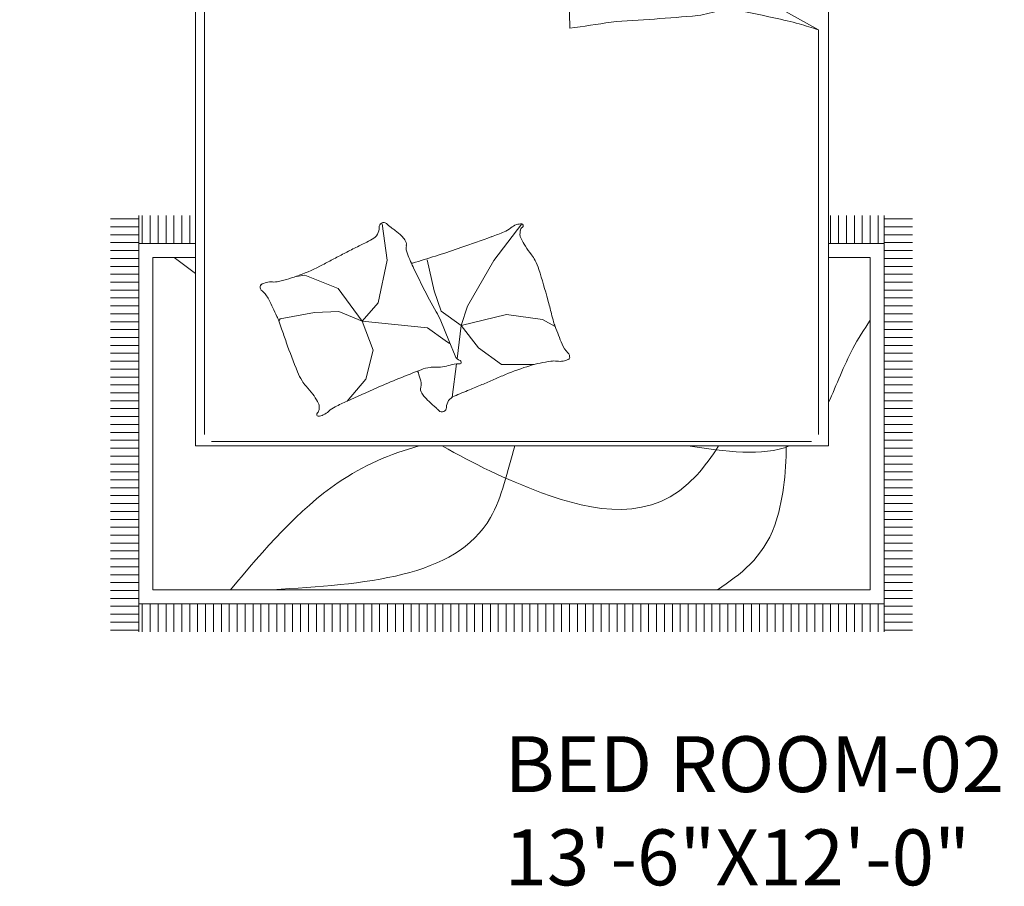
# Model space of a CAD drawing. Units: inches. Extents: x -7 to 1228, y -146 to 1091.
# Tile 52 of 88: x 74 to 163, y 885 to 964. Entities that reach past the tile are written whole.
import ezdxf

# ---------------------------------------------------------------- set-up
doc = ezdxf.new("R2010")
doc.units = ezdxf.units.IN
doc.layers.add('A-AREA-IDEN', color=7, linetype='Continuous', lineweight=18)
doc.layers.add('A-FURN', color=8, linetype='Continuous', lineweight=18)
doc.styles.add('DIM_FONT', font='SIMPLEX.shx', dxfattribs={"width": 0.8})
doc.styles.get("Standard").update_dxf_attribs({"font": 'arial.ttf'})

# ---------------------------------------------------------------- blocks, each defined once
blk = doc.blocks.new('A$C4F634EDD')
for p, q in [((0, 2.6295), (0, 2.2295)), ((0.5, 2.6295), (0, 2.6295)), ((0.5, 2.6295), (2.3, 2.6295)), ((0.5, 0.5295), (0.5, 2.6295)), ((0.5, 2.2295), (0.5, 2.6295)), ((2.3, 2.6295), (2.3, 0.5295)), ((2.3, 2.6295), (2.8, 2.6295)), ((2.3, 2.2295), (2.3, 2.6295)), ((2.8, 2.6295), (2.8, 2.2295)), ((0.5, 2.5771), (2.3, 2.5771)), ((2.392, 2.5115), (2.5692, 2.5765)), ((2.5692, 2.5765), (2.574, 2.5743)), ((0.2457, 2.5697), (0.2457, 2.4733)), ((2.4985, 2.5445), (2.5516, 2.564)), ((2.5062, 2.5454), (2.5487, 2.561)), ((2.5483, 2.5347), (2.5487, 2.561)), ((2.5487, 2.561), (2.5571, 2.56)), ((2.5615, 2.5536), (2.5514, 2.5318)), ((2.5516, 2.564), (2.5637, 2.5584)), ((2.5571, 2.56), (2.5615, 2.5536)), ((2.5615, 2.5536), (2.5791, 2.5058)), ((2.5637, 2.5584), (2.6418, 2.3458)), ((2.574, 2.5743), (2.6638, 2.3298)), ((2.4842, 2.5232), (2.47, 2.518)), ((2.4862, 2.5179), (2.4842, 2.5232)), ((2.4946, 2.5331), (2.4985, 2.5445)), ((2.5734, 2.3187), (2.4946, 2.5331)), ((2.5062, 2.5454), (2.5004, 2.5392)), ((2.5004, 2.5392), (2.5013, 2.5315)), ((2.5013, 2.5315), (2.5188, 2.4836)), ((2.5013, 2.5315), (2.5231, 2.5214)), ((2.5235, 2.5256), (2.5062, 2.5454)), ((2.5231, 2.5214), (2.5235, 2.5256)), ((2.5523, 2.4417), (2.5231, 2.5214)), ((2.5483, 2.5347), (2.5235, 2.5256)), ((2.5514, 2.5318), (2.5483, 2.5347)), ((2.5807, 2.4521), (2.5514, 2.5318)), ((2.3898, 2.5066), (2.392, 2.5115)), ((2.4795, 2.2621), (2.3898, 2.5066)), ((2.412, 2.5007), (2.4634, 2.5196)), ((2.4361, 2.4352), (2.412, 2.5007)), ((2.4634, 2.5196), (2.4875, 2.454)), ((2.47, 2.518), (2.472, 2.5127)), ((2.472, 2.5127), (2.4862, 2.5179)), ((2.4881, 2.5126), (2.4739, 2.5074)), ((2.4739, 2.5074), (2.4759, 2.502)), ((2.4759, 2.502), (2.4901, 2.5073)), ((2.492, 2.5019), (2.4778, 2.4967)), ((2.4778, 2.4967), (2.4798, 2.4914)), ((2.4798, 2.4914), (2.494, 2.4966)), ((2.4901, 2.5073), (2.4881, 2.5126)), ((2.494, 2.4966), (2.492, 2.5019)), ((2.5788, 2.4956), (2.5767, 2.4848)), ((2.5791, 2.5058), (2.5788, 2.4956)), ((2.4959, 2.4913), (2.4817, 2.4861)), ((2.4817, 2.4861), (2.4837, 2.4808)), ((2.4837, 2.4808), (2.4979, 2.486)), ((2.4998, 2.4807), (2.4856, 2.4755)), ((2.4856, 2.4755), (2.4876, 2.4702)), ((2.4876, 2.4702), (2.5018, 2.4754)), ((2.5037, 2.47), (2.4895, 2.4648)), ((2.4895, 2.4648), (2.4915, 2.4595)), ((2.4915, 2.4595), (2.5057, 2.4647)), ((2.4979, 2.486), (2.4959, 2.4913)), ((2.5018, 2.4754), (2.4998, 2.4807)), ((2.5057, 2.4647), (2.5037, 2.47)), ((2.5188, 2.4836), (2.5256, 2.4761)), ((2.5256, 2.4761), (2.5342, 2.4692)), ((2.5342, 2.4692), (2.5405, 2.4574)), ((2.5767, 2.4848), (2.5795, 2.4717)), ((2.5795, 2.4717), (2.586, 2.454)), ((2.4875, 2.454), (2.4361, 2.4352)), ((2.5405, 2.4574), (2.547, 2.4397)), ((2.5594, 2.4061), (2.547, 2.4397)), ((2.5523, 2.4417), (2.5875, 2.346)), ((2.5807, 2.4521), (2.6158, 2.3564)), ((2.5984, 2.4204), (2.586, 2.454)), ((0.0957, 2.4197), (0.192, 2.4197)), ((0.2994, 2.4197), (0.3957, 2.4197)), ((2.4457, 2.4146), (2.4563, 2.4185)), ((2.4496, 2.4039), (2.4457, 2.4146)), ((2.4563, 2.4185), (2.4602, 2.4078)), ((2.4634, 2.4211), (2.474, 2.425)), ((2.4673, 2.4104), (2.4634, 2.4211)), ((2.4779, 2.4143), (2.4673, 2.4104)), ((2.474, 2.425), (2.4779, 2.4143)), ((2.4811, 2.4276), (2.4917, 2.4315)), ((2.485, 2.4169), (2.4811, 2.4276)), ((2.4956, 2.4208), (2.485, 2.4169)), ((2.4883, 2.4081), (2.4989, 2.412)), ((2.4922, 2.3975), (2.4883, 2.4081)), ((2.4917, 2.4315), (2.4956, 2.4208)), ((2.4989, 2.412), (2.5028, 2.4014)), ((2.6047, 2.4086), (2.5984, 2.4204)), ((2.6133, 2.4017), (2.6047, 2.4086)), ((2.4602, 2.4078), (2.4496, 2.4039)), ((2.4528, 2.3951), (2.4635, 2.399)), ((2.4567, 2.3844), (2.4528, 2.3951)), ((2.4674, 2.3883), (2.4567, 2.3844)), ((2.4635, 2.399), (2.4674, 2.3883)), ((2.4706, 2.4016), (2.4812, 2.4055)), ((2.4745, 2.3909), (2.4706, 2.4016)), ((2.4851, 2.3949), (2.4745, 2.3909)), ((2.4777, 2.3821), (2.4883, 2.386)), ((2.4816, 2.3715), (2.4777, 2.3821)), ((2.4812, 2.4055), (2.4851, 2.3949)), ((2.4883, 2.386), (2.4922, 2.3754)), ((2.5028, 2.4014), (2.4922, 2.3975)), ((2.4954, 2.3886), (2.5061, 2.3925)), ((2.4993, 2.378), (2.4954, 2.3886)), ((2.51, 2.3819), (2.4993, 2.378)), ((2.5061, 2.3925), (2.51, 2.3819)), ((2.5238, 2.3769), (2.538, 2.3821)), ((2.538, 2.3821), (2.5419, 2.3715)), ((2.5622, 2.393), (2.5594, 2.4061)), ((2.5598, 2.372), (2.5601, 2.3822)), ((2.5601, 2.3822), (2.5622, 2.393)), ((2.6201, 2.3941), (2.6133, 2.4017)), ((2.6376, 2.3463), (2.6201, 2.3941)), ((2.6499, 2.3979), (2.6397, 2.3953)), ((2.6417, 2.39), (2.6488, 2.391)), ((2.6488, 2.391), (2.6538, 2.3895)), ((2.6551, 2.397), (2.6499, 2.3979)), ((2.6538, 2.3895), (2.6596, 2.388)), ((2.6627, 2.392), (2.6551, 2.397)), ((2.6596, 2.388), (2.6626, 2.3867)), ((2.6626, 2.3867), (2.6662, 2.388)), ((2.6692, 2.394), (2.6627, 2.392)), ((2.6662, 2.388), (2.6632, 2.3828)), ((2.6632, 2.3828), (2.6736, 2.3744)), ((2.6736, 2.3944), (2.6692, 2.394)), ((2.6765, 2.391), (2.6736, 2.3944)), ((2.6742, 2.3795), (2.6765, 2.391)), ((2.6824, 2.3858), (2.6742, 2.3795)), ((2.6873, 2.3815), (2.6824, 2.3858)), ((2.6853, 2.369), (2.6873, 2.3815)), ((0.2457, 2.366), (0.2457, 2.2697)), ((2.46, 2.3756), (2.4706, 2.3795)), ((2.4639, 2.365), (2.46, 2.3756)), ((2.4745, 2.3689), (2.4639, 2.365)), ((2.4672, 2.3561), (2.4778, 2.36)), ((2.4711, 2.3455), (2.4672, 2.3561)), ((2.4706, 2.3795), (2.4745, 2.3689)), ((2.4778, 2.36), (2.4817, 2.3494)), ((2.4922, 2.3754), (2.4816, 2.3715)), ((2.4849, 2.3626), (2.4955, 2.3665)), ((2.4888, 2.352), (2.4849, 2.3626)), ((2.4994, 2.3559), (2.4888, 2.352)), ((2.4955, 2.3665), (2.4994, 2.3559)), ((2.5026, 2.3691), (2.5132, 2.373)), ((2.5065, 2.3585), (2.5026, 2.3691)), ((2.5171, 2.3624), (2.5065, 2.3585)), ((2.5132, 2.373), (2.5171, 2.3624)), ((2.5277, 2.3663), (2.5238, 2.3769)), ((2.5419, 2.3715), (2.5277, 2.3663)), ((2.5774, 2.3242), (2.5598, 2.372)), ((2.6154, 2.3522), (2.5905, 2.3431)), ((2.6158, 2.3564), (2.6154, 2.3522)), ((2.6154, 2.3522), (2.6327, 2.3324)), ((2.6376, 2.3463), (2.6158, 2.3564)), ((2.6736, 2.3744), (2.6922, 2.3593)), ((2.6946, 2.376), (2.6853, 2.369)), ((2.6922, 2.3593), (2.7051, 2.3473)), ((2.6995, 2.3713), (2.6946, 2.376)), ((2.695, 2.3603), (2.6995, 2.3713)), ((2.7031, 2.3682), (2.695, 2.3603)), ((2.7096, 2.3616), (2.7031, 2.3682)), ((2.7062, 2.351), (2.7096, 2.3616)), ((2.7147, 2.3578), (2.7062, 2.351)), ((2.7214, 2.3517), (2.7147, 2.3578)), ((0, 2.3301), (0.5, 2.3301)), ((2.8, 2.3301), (2.3, 2.3301)), ((2.4817, 2.3494), (2.4711, 2.3455)), ((2.5774, 2.3242), (2.5875, 2.346)), ((2.5818, 2.3178), (2.5774, 2.3242)), ((2.5875, 2.346), (2.5905, 2.3431)), ((2.5905, 2.3431), (2.5901, 2.3168)), ((2.5901, 2.3168), (2.6097, 2.324)), ((2.613, 2.3312), (2.6077, 2.3293)), ((2.6077, 2.3293), (2.6135, 2.3141)), ((2.6192, 2.3174), (2.613, 2.3312)), ((2.6153, 2.3261), (2.6327, 2.3324)), ((2.6369, 2.332), (2.6161, 2.3243)), ((2.6616, 2.3249), (2.6234, 2.3109)), ((2.6327, 2.3324), (2.6385, 2.3386)), ((2.6418, 2.3458), (2.6369, 2.332)), ((2.6385, 2.3386), (2.6376, 2.3463)), ((2.6638, 2.3298), (2.6616, 2.3249)), ((2.7051, 2.3473), (2.7079, 2.3475)), ((2.7079, 2.3475), (2.7079, 2.3443)), ((2.7079, 2.3443), (2.727, 2.3277)), ((2.7196, 2.34), (2.7214, 2.3517)), ((2.7286, 2.3466), (2.7196, 2.34)), ((2.727, 2.3277), (2.7512, 2.2983)), ((2.7346, 2.3423), (2.7286, 2.3466)), ((2.732, 2.3295), (2.7346, 2.3423)), ((2.7423, 2.3345), (2.732, 2.3295)), ((2.7406, 2.3172), (2.7495, 2.325)), ((2.7495, 2.325), (2.7423, 2.3345)), ((2.6172, 2.3086), (2.4844, 2.2599)), ((2.5362, 2.305), (2.5185, 2.2985)), ((2.5185, 2.2985), (2.5224, 2.2879)), ((2.5401, 2.2944), (2.5362, 2.305)), ((2.561, 2.3141), (2.5433, 2.3076)), ((2.5433, 2.3076), (2.5472, 2.297)), ((2.5472, 2.297), (2.5649, 2.3035)), ((2.5649, 2.3035), (2.561, 2.3141)), ((2.5855, 2.3131), (2.5734, 2.3187)), ((2.5901, 2.3168), (2.5818, 2.3178)), ((2.6104, 2.3222), (2.5855, 2.3131)), ((2.6135, 2.3141), (2.6244, 2.2977)), ((2.626, 2.3069), (2.6192, 2.3174)), ((2.6244, 2.2977), (2.6349, 2.2825)), ((2.6365, 2.2916), (2.626, 2.3069)), ((2.7519, 2.3218), (2.7406, 2.3172)), ((2.7512, 2.2983), (2.756, 2.2695)), ((2.7575, 2.3144), (2.7519, 2.3218)), ((2.7526, 2.3045), (2.7575, 2.3144)), ((2.7622, 2.308), (2.7526, 2.3045)), ((2.7574, 2.2924), (2.7673, 2.2997)), ((2.7673, 2.2997), (2.7622, 2.308)), ((0.5953, 2.1912), (0.616, 2.2738)), ((1.4546, 2.1912), (1.4752, 2.2738)), ((2.5114, 2.2959), (2.4936, 2.2894)), ((2.4936, 2.2894), (2.4976, 2.2788)), ((2.4976, 2.2788), (2.5153, 2.2853)), ((2.5153, 2.2853), (2.5114, 2.2959)), ((2.5224, 2.2879), (2.5401, 2.2944)), ((2.6349, 2.2825), (2.638, 2.273)), ((2.6407, 2.2834), (2.6365, 2.2916)), ((2.6399, 2.2712), (2.6374, 2.2659)), ((2.638, 2.273), (2.6399, 2.2712)), ((2.6438, 2.2739), (2.6407, 2.2834)), ((2.6519, 2.2716), (2.6438, 2.2739)), ((2.6535, 2.2628), (2.6519, 2.2716)), ((2.756, 2.2695), (2.7459, 2.2483)), ((2.7687, 2.2905), (2.7574, 2.2924)), ((2.7587, 2.279), (2.7699, 2.2828)), ((2.7708, 2.2725), (2.7587, 2.279)), ((2.7699, 2.2828), (2.7687, 2.2905)), ((2.7706, 2.2643), (2.7708, 2.2725)), ((2.4844, 2.2599), (2.4795, 2.2621)), ((2.6374, 2.2659), (2.6398, 2.257)), ((2.6398, 2.257), (2.6509, 2.259)), ((2.6509, 2.259), (2.6431, 2.2492)), ((2.6431, 2.2492), (2.6473, 2.2398)), ((2.6473, 2.2398), (2.6592, 2.2429)), ((2.6592, 2.2429), (2.6521, 2.2314)), ((2.6636, 2.2409), (2.6535, 2.2628)), ((2.6836, 2.2287), (2.6636, 2.2409)), ((2.7459, 2.2483), (2.7284, 2.2317)), ((2.7509, 2.2314), (2.7459, 2.2418)), ((2.7459, 2.2418), (2.7568, 2.2352)), ((2.7529, 2.2505), (2.7645, 2.2498)), ((2.7607, 2.2424), (2.7529, 2.2505)), ((2.7568, 2.2352), (2.7607, 2.2424)), ((2.759, 2.2637), (2.7706, 2.2643)), ((2.7676, 2.2559), (2.759, 2.2637)), ((2.7645, 2.2498), (2.7676, 2.2559)), ((0, 2.2295), (0.5, 2.2295)), ((2.8, 2.2295), (2.3, 2.2295)), ((2.6521, 2.2314), (2.6598, 2.2248)), ((2.6598, 2.2248), (2.6697, 2.2309)), ((2.6697, 2.2309), (2.6684, 2.219)), ((2.6684, 2.219), (2.6761, 2.2145)), ((2.6761, 2.2145), (2.6821, 2.2237)), ((2.6821, 2.2237), (2.6843, 2.2135)), ((2.7063, 2.2256), (2.6836, 2.2287)), ((2.6843, 2.2135), (2.6927, 2.2117)), ((2.6927, 2.2117), (2.6986, 2.222)), ((2.6986, 2.222), (2.7019, 2.2098)), ((2.7284, 2.2317), (2.7063, 2.2256)), ((2.7102, 2.2104), (2.7113, 2.2218)), ((2.7113, 2.2218), (2.7192, 2.2137)), ((2.7192, 2.2137), (2.7255, 2.2152)), ((2.7255, 2.2152), (2.7242, 2.2265)), ((2.7242, 2.2265), (2.7324, 2.2165)), ((2.7324, 2.2165), (2.7386, 2.2208)), ((2.7386, 2.2208), (2.7354, 2.2306)), ((2.7354, 2.2306), (2.7462, 2.2264)), ((2.7462, 2.2264), (2.7509, 2.2314)), ((0.5878, 2.1612), (0.5953, 2.1912)), ((1.4471, 2.1612), (1.4546, 2.1912)), ((2.7019, 2.2098), (2.7102, 2.2104)), ((1.5035, 2.141), (0.5458, 2.141)), ((1.5035, 2.141), (2.2716, 1.7136)), ((0.5258, 2.121), (0.5258, 0.5617)), ((1.576, 1.9433), (1.5624, 1.8479)), ((0.5458, 1.8684), (1.5653, 1.8684)), ((1.5624, 1.8479), (1.5641, 1.7178)), ((2.2716, 0.5617), (2.2716, 1.7136)), ((0.3386, 0), (0.3386, 1.1852)), ((0.3486, 1.1052), (0.3486, 1.1852)), ((0.3711, 1.1052), (0.3711, 1.1852)), ((0.3936, 1.1052), (0.3936, 1.1852)), ((0.4161, 1.1052), (0.4161, 1.1852)), ((0.4386, 1.1052), (0.4386, 1.1852)), ((0.4611, 1.1052), (0.4611, 1.1852)), ((0.4836, 1.1052), (0.4836, 1.1852)), ((2.3061, 1.1052), (2.3061, 1.1852)), ((2.3286, 1.1052), (2.3286, 1.1852)), ((2.3511, 1.1052), (2.3511, 1.1852)), ((2.3736, 1.1052), (2.3736, 1.1852)), ((2.3961, 1.1052), (2.3961, 1.1852)), ((2.4186, 1.1052), (2.4186, 1.1852)), ((2.4411, 1.1052), (2.4411, 1.1852)), ((2.4588, 1.1852), (2.4588, 0)), ((0.2586, 1.1753), (0.3386, 1.1753)), ((0.2586, 1.1528), (0.3386, 1.1528)), ((1.031, 1.1612), (1.0448, 1.0581)), ((1.4276, 1.1611), (1.3484, 1.0571)), ((2.4588, 1.1753), (2.5388, 1.1753)), ((2.4588, 1.1528), (2.5388, 1.1528)), ((0.2586, 1.1303), (0.3386, 1.1303)), ((2.4588, 1.1303), (2.5388, 1.1303)), ((0.2586, 1.1078), (0.3386, 1.1078)), ((0.3386, 1.1052), (0.5, 1.1052)), ((2.3, 1.1052), (2.4588, 1.1052)), ((2.4588, 1.1078), (2.5388, 1.1078)), ((0.2586, 1.0853), (0.3386, 1.0853)), ((0.3786, 1.0652), (0.5, 1.0652)), ((0.3786, 0.12), (0.3786, 1.0652)), ((2.3, 1.0652), (2.4188, 1.0652)), ((2.4188, 1.0652), (2.4188, 0.12)), ((2.4588, 1.0853), (2.5388, 1.0853)), ((0.2586, 1.0628), (0.3386, 1.0628)), ((0.2586, 1.0403), (0.3386, 1.0403)), ((1.0448, 1.0581), (1.019, 0.936)), ((1.1784, 0.9702), (1.1586, 1.0591)), ((1.3484, 1.0571), (1.2733, 0.9268)), ((2.4588, 1.0628), (2.5388, 1.0628)), ((2.4588, 1.0403), (2.5388, 1.0403)), ((0.2586, 1.0178), (0.3386, 1.0178)), ((0.8108, 1.0151), (0.7868, 1.0117)), ((0.9054, 0.9773), (0.8108, 1.0151)), ((2.4588, 1.0178), (2.5388, 1.0178)), ((0.2586, 0.9953), (0.3386, 0.9953)), ((2.4588, 0.9953), (2.5388, 0.9953)), ((0.2586, 0.9728), (0.3386, 0.9728)), ((0.9743, 0.8845), (0.9054, 0.9773)), ((1.1982, 0.9129), (1.1784, 0.9702)), ((2.4588, 0.9728), (2.5388, 0.9728)), ((0.2586, 0.9503), (0.3386, 0.9503)), ((0.2586, 0.9278), (0.3386, 0.9278)), ((1.019, 0.936), (0.9743, 0.8845)), ((1.2733, 0.9268), (1.2555, 0.8715)), ((2.4588, 0.9503), (2.5388, 0.9503)), ((2.4588, 0.9278), (2.5388, 0.9278)), ((0.2586, 0.9053), (0.3386, 0.9053)), ((0.8384, 0.9085), (0.7403, 0.8913)), ((0.9072, 0.912), (0.8384, 0.9085)), ((0.9743, 0.8845), (0.9072, 0.912)), ((1.2555, 0.8715), (1.1982, 0.9129)), ((1.2555, 0.8715), (1.384, 0.9031)), ((1.384, 0.9031), (1.4868, 0.8892)), ((2.4588, 0.9053), (2.5388, 0.9053)), ((0.2586, 0.8828), (0.3386, 0.8828)), ((0.7403, 0.8913), (0.737, 0.8849)), ((0.9743, 0.8845), (1.0052, 0.802)), ((0.9743, 0.8845), (1.16, 0.8656)), ((1.1973, 0.8853), (1.2203, 0.829)), ((1.2555, 0.8715), (1.2437, 0.7773)), ((1.2555, 0.8715), (1.3049, 0.8082)), ((1.4868, 0.8892), (1.5228, 0.8692)), ((2.4588, 0.8828), (2.5388, 0.8828)), ((0.2586, 0.8603), (0.3386, 0.8603)), ((1.16, 0.8656), (1.2099, 0.8295)), ((2.4588, 0.8603), (2.5388, 0.8603)), ((0.2586, 0.8378), (0.3386, 0.8378)), ((0.2586, 0.8153), (0.3386, 0.8153)), ((1.2099, 0.8295), (1.222, 0.8209)), ((1.2203, 0.829), (1.2381, 0.7855)), ((2.4588, 0.8378), (2.5388, 0.8378)), ((2.4588, 0.8153), (2.5388, 0.8153)), ((0.2586, 0.7928), (0.3386, 0.7928)), ((1.0052, 0.802), (0.9846, 0.7194)), ((1.3049, 0.8082), (1.3701, 0.7608)), ((2.4588, 0.7928), (2.5388, 0.7928)), ((0.2586, 0.7703), (0.3386, 0.7703)), ((1.2419, 0.7626), (1.23, 0.668)), ((1.3701, 0.7608), (1.463, 0.7608)), ((2.4588, 0.7703), (2.5388, 0.7703)), ((0.2586, 0.7478), (0.3386, 0.7478)), ((2.4588, 0.7478), (2.5388, 0.7478)), ((0.2586, 0.7253), (0.3386, 0.7253)), ((0.2586, 0.7028), (0.3386, 0.7028)), ((0.9846, 0.7194), (0.931, 0.6569)), ((2.4588, 0.7253), (2.5388, 0.7253)), ((2.4588, 0.7028), (2.5388, 0.7028)), ((0.2586, 0.6803), (0.3386, 0.6803)), ((2.4588, 0.6803), (2.5388, 0.6803)), ((0.2586, 0.6578), (0.3386, 0.6578)), ((2.4588, 0.6578), (2.5388, 0.6578)), ((0.2586, 0.6353), (0.3386, 0.6353)), ((2.4588, 0.6353), (2.5388, 0.6353)), ((0.2586, 0.6128), (0.3386, 0.6128)), ((0.2586, 0.5903), (0.3386, 0.5903)), ((2.4588, 0.6128), (2.5388, 0.6128)), ((2.4588, 0.5903), (2.5388, 0.5903)), ((0.2586, 0.5678), (0.3386, 0.5678)), ((2.4588, 0.5678), (2.5388, 0.5678)), ((0.2586, 0.5453), (0.3386, 0.5453)), ((0.5458, 0.5417), (2.2516, 0.5417)), ((2.4588, 0.5453), (2.5388, 0.5453)), ((0.2586, 0.5228), (0.3386, 0.5228)), ((2.3, 0.5295), (0.5, 0.5295)), ((2.4588, 0.5228), (2.5388, 0.5228)), ((0.2586, 0.5003), (0.3386, 0.5003)), ((0.2586, 0.4778), (0.3386, 0.4778)), ((2.4588, 0.5003), (2.5388, 0.5003)), ((2.4588, 0.4778), (2.5388, 0.4778)), ((0.2586, 0.4553), (0.3386, 0.4553)), ((2.4588, 0.4553), (2.5388, 0.4553)), ((0.2586, 0.4328), (0.3386, 0.4328)), ((2.4588, 0.4328), (2.5388, 0.4328)), ((0.2586, 0.4103), (0.3386, 0.4103)), ((2.4588, 0.4103), (2.5388, 0.4103)), ((0.2586, 0.3878), (0.3386, 0.3878)), ((0.2586, 0.3653), (0.3386, 0.3653)), ((2.4588, 0.3878), (2.5388, 0.3878)), ((2.4588, 0.3653), (2.5388, 0.3653)), ((0.2586, 0.3428), (0.3386, 0.3428)), ((2.4588, 0.3428), (2.5388, 0.3428)), ((0.2586, 0.3203), (0.3386, 0.3203)), ((2.4588, 0.3203), (2.5388, 0.3203)), ((0.2586, 0.2978), (0.3386, 0.2978)), ((2.4588, 0.2978), (2.5388, 0.2978)), ((0.2586, 0.2753), (0.3386, 0.2753)), ((0.2586, 0.2528), (0.3386, 0.2528)), ((2.4588, 0.2753), (2.5388, 0.2753)), ((2.4588, 0.2528), (2.5388, 0.2528)), ((0.2586, 0.2303), (0.3386, 0.2303)), ((2.4588, 0.2303), (2.5388, 0.2303)), ((0.2586, 0.2078), (0.3386, 0.2078)), ((2.4588, 0.2078), (2.5388, 0.2078)), ((0.2586, 0.1853), (0.3386, 0.1853)), ((2.4588, 0.1853), (2.5388, 0.1853)), ((0.2586, 0.1628), (0.3386, 0.1628)), ((0.2586, 0.1403), (0.3386, 0.1403)), ((2.4588, 0.1628), (2.5388, 0.1628)), ((2.4588, 0.1403), (2.5388, 0.1403)), ((0.2586, 0.1178), (0.3386, 0.1178)), ((2.4188, 0.12), (0.3786, 0.12)), ((2.4588, 0.1178), (2.5388, 0.1178)), ((0.2586, 0.0953), (0.3386, 0.0953)), ((2.4588, 0.0953), (2.5388, 0.0953)), ((0.2586, 0.0728), (0.3386, 0.0728)), ((2.4588, 0.08), (0.3386, 0.08)), ((0.3486, 0), (0.3486, 0.08)), ((0.3711, 0), (0.3711, 0.08)), ((0.3936, 0), (0.3936, 0.08)), ((0.4161, 0), (0.4161, 0.08)), ((0.4386, 0), (0.4386, 0.08)), ((0.4611, 0), (0.4611, 0.08)), ((0.4836, 0), (0.4836, 0.08)), ((0.5061, 0), (0.5061, 0.08)), ((0.5286, 0), (0.5286, 0.08)), ((0.5511, 0), (0.5511, 0.08)), ((0.5736, 0), (0.5736, 0.08)), ((0.5961, 0), (0.5961, 0.08)), ((0.6186, 0), (0.6186, 0.08)), ((0.6411, 0), (0.6411, 0.08)), ((0.6636, 0), (0.6636, 0.08)), ((0.6861, 0), (0.6861, 0.08)), ((0.7086, 0), (0.7086, 0.08)), ((0.7311, 0), (0.7311, 0.08)), ((0.7536, 0), (0.7536, 0.08)), ((0.7761, 0), (0.7761, 0.08)), ((0.7986, 0), (0.7986, 0.08)), ((0.8211, 0), (0.8211, 0.08)), ((0.8436, 0), (0.8436, 0.08)), ((0.8661, 0), (0.8661, 0.08)), ((0.8886, 0), (0.8886, 0.08)), ((0.9111, 0), (0.9111, 0.08)), ((0.9336, 0), (0.9336, 0.08)), ((0.9561, 0), (0.9561, 0.08)), ((0.9786, 0), (0.9786, 0.08)), ((1.0011, 0), (1.0011, 0.08)), ((1.0236, 0), (1.0236, 0.08)), ((1.0461, 0), (1.0461, 0.08)), ((1.0686, 0), (1.0686, 0.08)), ((1.0911, 0), (1.0911, 0.08)), ((1.1136, 0), (1.1136, 0.08)), ((1.1361, 0), (1.1361, 0.08)), ((1.1586, 0), (1.1586, 0.08)), ((1.1811, 0), (1.1811, 0.08)), ((1.2036, 0), (1.2036, 0.08)), ((1.2261, 0), (1.2261, 0.08)), ((1.2486, 0), (1.2486, 0.08)), ((1.2711, 0), (1.2711, 0.08)), ((1.2936, 0), (1.2936, 0.08)), ((1.3161, 0), (1.3161, 0.08)), ((1.3386, 0), (1.3386, 0.08)), ((1.3611, 0), (1.3611, 0.08)), ((1.3836, 0), (1.3836, 0.08)), ((1.4061, 0), (1.4061, 0.08)), ((1.4286, 0), (1.4286, 0.08)), ((1.4511, 0), (1.4511, 0.08)), ((1.4736, 0), (1.4736, 0.08)), ((1.4961, 0), (1.4961, 0.08)), ((1.5186, 0), (1.5186, 0.08)), ((1.5411, 0), (1.5411, 0.08)), ((1.5636, 0), (1.5636, 0.08)), ((1.5861, 0), (1.5861, 0.08)), ((1.6086, 0), (1.6086, 0.08)), ((1.6311, 0), (1.6311, 0.08)), ((1.6536, 0), (1.6536, 0.08)), ((1.6761, 0), (1.6761, 0.08)), ((1.6986, 0), (1.6986, 0.08)), ((1.7211, 0), (1.7211, 0.08)), ((1.7436, 0), (1.7436, 0.08)), ((1.7661, 0), (1.7661, 0.08)), ((1.7886, 0), (1.7886, 0.08)), ((1.8111, 0), (1.8111, 0.08)), ((1.8336, 0), (1.8336, 0.08)), ((1.8561, 0), (1.8561, 0.08)), ((1.8786, 0), (1.8786, 0.08)), ((1.9011, 0), (1.9011, 0.08)), ((1.9236, 0), (1.9236, 0.08)), ((1.9461, 0), (1.9461, 0.08)), ((1.9686, 0), (1.9686, 0.08)), ((1.9911, 0), (1.9911, 0.08)), ((2.0136, 0), (2.0136, 0.08)), ((2.0361, 0), (2.0361, 0.08)), ((2.0586, 0), (2.0586, 0.08)), ((2.0811, 0), (2.0811, 0.08)), ((2.1036, 0), (2.1036, 0.08)), ((2.1261, 0), (2.1261, 0.08)), ((2.1486, 0), (2.1486, 0.08)), ((2.1711, 0), (2.1711, 0.08)), ((2.1936, 0), (2.1936, 0.08)), ((2.2161, 0), (2.2161, 0.08)), ((2.2386, 0), (2.2386, 0.08)), ((2.2611, 0), (2.2611, 0.08)), ((2.2836, 0), (2.2836, 0.08)), ((2.3061, 0), (2.3061, 0.08)), ((2.3286, 0), (2.3286, 0.08)), ((2.3511, 0), (2.3511, 0.08)), ((2.3736, 0), (2.3736, 0.08)), ((2.3961, 0), (2.3961, 0.08)), ((2.4186, 0), (2.4186, 0.08)), ((2.4411, 0), (2.4411, 0.08)), ((2.4588, 0.0728), (2.5388, 0.0728)), ((0.2586, 0.0503), (0.3386, 0.0503)), ((2.4588, 0.0503), (2.5388, 0.0503)), ((0.2586, 0.0278), (0.3386, 0.0278)), ((0.2586, 0.0053), (0.3386, 0.0053)), ((2.4588, 0.0278), (2.5388, 0.0278)), ((2.4588, 0.0053), (2.5388, 0.0053))]:
    blk.add_line(p, q)
for radius in [0.1222, 0.0865]:
    blk.add_circle((0.2457, 2.4197), radius)
for centre, radius, start, end in [((0.5848, 2.5274), 0.0131, 101.2724, 206.5805), ((0.6036, 2.5368), 0.0342, 206.5805, 265.5998), ((0.5999, 2.4516), 0.0904, 90, 101.2724), ((0.5999, 2.3808), 0.1611, 81.5628, 90), ((0.5788, 2.2388), 0.3048, 74.256, 81.5628), ((0.7272, 2.7653), 0.2422, 254.256, 262.4531), ((0.7851, 3.2019), 0.6827, 262.4531, 270), ((0.7851, 3.5682), 1.049, 270, 276.0867), ((0.8402, 3.0514), 0.5293, 276.0867, 280.1899), ((1.1602, -8.1346), 10.6675, 90.30153, 91.21582), ((1.1169, 2.2433), 0.2897, 85.1982, 92.5386), ((1.2142, 3.4021), 0.8732, 265.1982, 269.4243), ((1.3082, 2.3102), 0.234, 110.8603, 117.2396), ((1.2204, 4.0232), 1.4943, 269.4243, 271.9079), ((1.2995, 2.4357), 0.0992, 105.9352, 126.0864), ((1.2429, 3.3501), 0.8208, 271.9079, 275.2592), ((1.2995, 2.4357), 0.0992, 85.7841, 105.9352), ((1.3132, 2.5864), 0.0539, 275.2592, 300.6513), ((1.3554, 2.5152), 0.0289, 85.6975, 120.6513), ((1.3556, 2.519), 0.0251, 68.2117, 85.6975), ((1.3739, 2.5288), 0.0156, 158.0096, 201.421), ((1.3634, 2.533), 0.00428, 78.1069, 158.0096), ((1.3288, 2.5111), 0.0328, 351.8665, 21.421), ((1.3647, 2.5395), 0.00232, 258.1069, 19.564), ((1.3637, 2.5391), 0.00342, 19.564, 68.2117), ((1.444, 2.5274), 0.0131, 101.2724, 206.5805), ((1.4628, 2.5368), 0.0342, 206.5805, 265.5998), ((1.4591, 2.4516), 0.0904, 90, 101.2724), ((1.4591, 2.3808), 0.1611, 81.5628, 90), ((1.438, 2.2388), 0.3048, 74.256, 81.5628), ((1.5865, 2.7653), 0.2422, 254.256, 262.4531), ((1.6443, 3.2019), 0.6827, 262.4531, 270), ((1.6443, 3.5682), 1.049, 270, 276.0867), ((1.4785, 15.4878), 12.9656, 271.22425, 272.05324), ((1.97, 2.3805), 0.1524, 92.5386, 100.1899), ((1.9761, 2.2433), 0.2897, 85.1982, 92.5386), ((2.0734, 3.4021), 0.8732, 265.1982, 269.4243), ((2.1674, 2.3102), 0.234, 110.8603, 117.2396), ((2.0797, 4.0232), 1.4943, 269.4243, 271.9079), ((2.1588, 2.4357), 0.0992, 105.9352, 126.0864), ((2.1021, 3.3501), 0.8208, 271.9079, 275.2592), ((2.1588, 2.4357), 0.0992, 85.7841, 105.9352), ((2.1724, 2.5864), 0.0539, 275.2592, 300.6513), ((2.2146, 2.5152), 0.0289, 85.6975, 120.6513), ((2.2149, 2.519), 0.0251, 68.2117, 85.6975), ((2.2331, 2.5288), 0.0156, 158.0096, 201.421), ((2.2226, 2.533), 0.00428, 78.1069, 158.0096), ((2.1881, 2.5111), 0.0328, 351.8665, 21.421), ((2.224, 2.5395), 0.00232, 258.1069, 19.564), ((2.2229, 2.5391), 0.00342, 19.564, 68.2117), ((1.0898, 2.4496), 0.4918, 173.7676, 180), ((0.5368, 2.3783), 0.1399, 45.0976, 62.7964), ((1.4317, 2.2032), 0.3916, 128.3886, 133.8115), ((1.2362, 2.45), 0.0768, 117.2396, 128.3886), ((1.2995, 2.4357), 0.0992, 143.8234, 161.5603), ((1.2995, 2.4357), 0.0992, 126.0864, 143.8234), ((1.1177, 2.5413), 0.246, 347.8905, 351.8665), ((1.949, 2.4496), 0.4918, 173.7676, 180), ((2.291, 2.2032), 0.3916, 128.3886, 133.8115), ((2.0954, 2.45), 0.0768, 117.2396, 128.3886), ((2.1588, 2.4357), 0.0992, 143.8234, 161.5603), ((2.1588, 2.4357), 0.0992, 126.0864, 143.8234), ((1.977, 2.5413), 0.246, 347.8905, 351.8665), ((0.5462, 2.4142), 0.0899, 41.4429, 53.7359), ((0.5741, 2.4389), 0.0526, 25.3551, 41.4429), ((0.5368, 2.3783), 0.1399, 27.3988, 45.0976), ((1.1799, 2.4341), 0.0493, 140.9651, 151.6832), ((1.3165, 2.3233), 0.2252, 133.8115, 140.9651), ((2.2605, 2.3525), 0.9131, 172.3191, 176.6313), ((1.5522, 2.448), 0.1983, 167.8905, 172.3191), ((2.0391, 2.4341), 0.0493, 140.9651, 151.6832), ((2.1757, 2.3233), 0.2252, 133.8115, 140.9651), ((3.1198, 2.3525), 0.9131, 172.3191, 176.6313), ((2.4114, 2.448), 0.1983, 167.8905, 172.3191), ((0.8019, 2.4496), 0.204, 180, 189.6844), ((0.4851, 2.3967), 0.1511, 21.8149, 25.3551), ((0.4345, 2.3765), 0.2056, 18.7799, 21.8149), ((0.576, 2.4246), 0.0562, 0, 18.7799), ((0.5368, 2.3783), 0.1399, 16.515, 27.3988), ((1.3127, 2.3625), 0.2002, 151.6832, 156.9972), ((1.6611, 2.4496), 0.204, 180, 189.6844), ((2.1719, 2.3625), 0.2002, 151.6832, 156.9972), ((1.4703, 2.5637), 0.882, 189.6844, 192.1984), ((0.5406, 2.4246), 0.0915, 345.3149, 0), ((0.5368, 2.3783), 0.1399, 5.6311, 16.515), ((2.3295, 2.5637), 0.882, 189.6844, 192.1984), ((2.0266, 2.3663), 0.6787, 176.6313, 181.6331), ((2.8858, 2.3663), 0.6787, 176.6313, 181.6331), ((0.2982, 2.3103), 0.3171, 8.0051, 12.1984), ((-0.0401, 2.2627), 0.6588, 2.6649, 8.0051), ((1.1575, 2.3103), 0.3171, 8.0051, 12.1984), ((0.8191, 2.2627), 0.6588, 2.6649, 8.0051), ((2.7128, 2.3859), 1.3652, 181.6331, 183.055), ((3.5721, 2.3859), 1.3652, 181.6331, 183.055), ((14.9657, 3.0398), 13.6356, 183.05496, 183.50486), ((15.8249, 3.0398), 13.6356, 183.05496, 183.50486), ((0.5503, 2.2902), 0.0677, 345.9548, 2.6649), ((1.4096, 2.2902), 0.0677, 345.9548, 2.6649), ((1.1303, 1.9835), 0.2721, 85.9172, 93.5552), ((1.1455, 2.197), 0.058, 69.3257, 85.9172), ((0.9871, 1.7772), 0.5066, 65.6735, 69.3257), ((0.473, 2.8815), 0.7387, 293.4844, 295.3111), ((0.6058, 0.9338), 1.4323, 63.5015, 65.6735), ((1.1054, 1.9358), 0.3126, 57.865, 63.5015), ((1.3322, 2.8815), 0.7387, 293.4844, 295.3111), ((0.473, 2.8815), 0.7387, 287.1982, 289.428), ((0.473, 2.8815), 0.7387, 289.428, 291.6577), ((0.473, 2.8815), 0.7387, 291.6577, 293.4844), ((0.8841, 1.5835), 0.7286, 54.1737, 57.865), ((1.6762, 2.2258), 0.3212, 183.5049, 189.9984), ((1.3322, 2.8815), 0.7387, 287.1982, 289.428), ((1.3322, 2.8815), 0.7387, 289.428, 291.6577), ((1.3322, 2.8815), 0.7387, 291.6577, 293.4844), ((2.5355, 2.2258), 0.3212, 183.5049, 189.9984), ((0.5887, 2.1609), 0.000917, 165.9551, 274.0829), ((0.5695, 2.4301), 0.2708, 274.0829, 279.4841), ((0.5763, 2.3896), 0.2297, 279.4841, 287.3864), ((0.6807, 2.0561), 0.1197, 96.4341, 107.3864), ((0.6836, 2.0301), 0.1459, 78.4414, 96.4341), ((0.759, 2.3985), 0.2301, 258.4414, 272.7491), ((0.7026, 3.5718), 1.4048, 272.7491, 274.6176), ((0.9136, 0.9591), 1.2165, 92.6096, 94.6176), ((1.2501, -19.8405), 22.0183, 90.37908, 91.01965), ((1.2012, -3.5404), 5.7185, 89.7135, 90.9704), ((1.224, 1.0141), 1.164, 86.426, 89.7135), ((1.2875, 2.0302), 0.1459, 77.131, 86.426), ((1.3099, 2.1283), 0.0453, 62.7159, 77.131), ((1.3658, 2.2367), 0.0767, 242.7159, 253.7788), ((1.3688, 2.247), 0.0875, 253.7788, 262.8796), ((1.3581, 2.1615), 0.00132, 262.8796, 343.3022), ((1.3409, 2.1667), 0.0193, 343.3022, 9.9984), ((1.448, 2.1609), 0.000917, 165.9551, 274.0829), ((1.4288, 2.4301), 0.2708, 274.0829, 279.4841), ((1.4355, 2.3896), 0.2297, 279.4841, 287.3864), ((1.5399, 2.0561), 0.1197, 96.4341, 107.3864), ((1.5429, 2.0301), 0.1459, 78.4414, 96.4341), ((1.6182, 2.3985), 0.2301, 258.4414, 272.7491), ((1.5619, 3.5718), 1.4048, 272.7491, 274.6176), ((1.7729, 0.9591), 1.2165, 92.6096, 94.6176), ((2.1093, -19.8405), 22.0183, 90.37908, 91.01965), ((2.0605, -3.5404), 5.7185, 89.7135, 90.9704), ((2.0833, 1.0141), 1.164, 86.426, 89.7135), ((2.1467, 2.0302), 0.1459, 77.131, 86.426), ((2.1691, 2.1283), 0.0453, 62.7159, 77.131), ((2.2251, 2.2367), 0.0767, 242.7159, 253.7788), ((2.2281, 2.247), 0.0875, 253.7788, 262.8796), ((2.2174, 2.1615), 0.00132, 262.8796, 343.3022), ((2.2001, 2.1667), 0.0193, 343.3022, 9.9984), ((0.5458, 2.121), 0.02, 90, 180), ((1.2147, 1.9017), 0.3751, 20.1488, 39.6445), ((1.3977, 1.9688), 0.1801, 351.8644, 20.1488), ((0.5458, 1.8884), 0.02, 180, 270), ((1.4194, 4.2174), 2.5158, 281.6741, 283.1904), ((2.0378, 1.5789), 0.1942, 97.7304, 103.1904), ((2.0195, 1.7137), 0.0581, 79.2724, 97.7304), ((1.2737, -2.2227), 4.0646, 77.0745, 79.2724), ((0.6102, 18.0525), 16.3521, 273.75703, 274.62393), ((2.0359, 1.0981), 0.6574, 74.0648, 77.0745), ((1.0582, 5.4638), 3.7801, 277.692, 279.495), ((1.7125, -0.0344), 1.8351, 72.2636, 74.0648), ((0.9863, 1.1494), 0.0359, 297.2902, 3.2455), ((1.0348, 1.1521), 0.0127, 51.1864, 183.2455), ((0.9991, 1.1077), 0.0697, 45.8726, 51.1864), ((1.0791, 1.1902), 0.0452, 225.8726, 232.4713), ((1.2846, 1.4577), 0.3825, 232.4713, 233.7837), ((0.6683, 0.6162), 0.6605, 52.7849, 53.7837), ((1.3469, 1.2115), 0.0792, 292.7069, 308.5854), ((1.4338, 1.1026), 0.0601, 110.3452, 128.5854), ((1.4251, 1.1259), 0.0352, 86.0516, 110.3452), ((1.4376, 1.1398), 0.0142, 126.5792, 169.5926), ((1.4273, 1.1567), 0.00443, 13.2808, 86.0516), ((1.4254, 1.1562), 0.0063, 306.5792, 13.2808), ((0.9362, 0.9689), 0.2176, 46.4776, 52.7849), ((1.0327, 1.0706), 0.0774, 35.8936, 46.4776), ((-0.4107, 5.9078), 5.0942, 289.0836, 290.1287), ((1.0543, 1.9106), 0.8371, 290.1287, 292.7069), ((1.4996, 1.1284), 0.0771, 169.5926, 177.2714), ((1.4378, 1.1314), 0.0153, 177.2714, 194.5709), ((1.4611, 1.1374), 0.0393, 194.5709, 206.8179), ((1.8575, -0.7096), 2.0162, 116.4147, 117.4999), ((-0.4173, 3.8699), 3.0972, 296.4147, 297.2902), ((1.0771, 1.1027), 0.0226, 351.9508, 35.8936), ((1.1449, 1.0931), 0.0458, 171.9508, 202.4162), ((0.2266, 4.0657), 3.145, 286.6085, 289.0836), ((1.7401, 1.2785), 0.352, 206.8179, 210.9056), ((1.6045, 1.1973), 0.194, 210.9056, 219.7005), ((3.744, -4.3336), 6.1019, 117.49986, 117.84822), ((2.032, 1.4591), 1.0054, 202.4162, 205.0529), ((1.3929, 1.0217), 0.081, 26.0735, 39.7005), ((0.5736, 1.5979), 0.6236, 290.7486, 297.4921), ((-1.8336, 6.2238), 5.8383, 297.49208, 297.84822), ((1.0922, 1.1636), 0.1166, 280.7366, 286.6085), ((1.2892, 0.9709), 0.1965, 17.8396, 26.0735), ((0.6422, 1.4168), 0.43, 282.6252, 290.7486), ((2.6493, 1.7476), 1.6868, 205.0529, 207.0884), ((-0.4304, 0.4175), 2.003, 15.2625, 17.8396), ((0.6894, 0.9832), 0.0058, 121.6917, 179.0386), ((0.7004, 0.983), 0.0168, 179.0386, 229.4914), ((0.7131, 0.9448), 0.0509, 103.0402, 121.6917), ((0.7152, 0.9361), 0.0599, 86.6119, 103.0402), ((0.7224, 1.0587), 0.063, 266.6119, 282.6252), ((0.6405, 0.9128), 0.0755, 26.3332, 49.4914), ((2.541, 1.6922), 1.5652, 207.0884, 209.936), ((-1.6775, -0.2344), 2.6619, 25.1732, 26.3332), ((-0.0881, 0.5109), 1.6481, 13.841, 15.2625), ((0.5689, 0.8213), 0.1798, 20.7081, 25.1732), ((0.9989, 0.8042), 0.2143, 22.2355, 29.936), ((2.0418, 1.0357), 0.5454, 193.841, 196.3122), ((0.2268, 0.692), 0.5454, 18.2369, 20.7081), ((1.6908, 0.933), 0.1798, 196.3122, 200.7773), ((4.0115, 1.8135), 2.6619, 200.7773, 201.9373), ((2.3102, 1.3785), 1.6481, 198.2369, 199.6584), ((2.6444, 1.4979), 2.003, 199.6584, 202.2355), ((1.6124, 0.8472), 0.0755, 201.9373, 225.0955), ((1.2594, 0.7942), 0.0231, 202.2355, 252.8133), ((1.5473, 0.7819), 0.0168, 354.6428, 45.0955), ((1.1727, 0.9313), 0.1794, 277.6784, 284.8807), ((1.2689, 0.569), 0.1955, 97.9822, 104.8807), ((1.2465, 0.729), 0.034, 85.7407, 97.9822), ((1.2497, 0.772), 0.0092, 265.7407, 289.3799), ((1.2512, 0.7678), 0.00467, 289.3799, 72.8133), ((1.6266, 0.159), 0.6236, 106.3527, 113.0962), ((1.5721, 0.3449), 0.43, 98.2293, 106.3527), ((1.5195, 0.708), 0.063, 82.216, 98.2293), ((1.5362, 0.8298), 0.0599, 262.216, 278.6443), ((1.5375, 0.8209), 0.0509, 278.6443, 297.2959), ((1.5582, 0.7808), 0.0058, 297.2959, 354.6428), ((0.9722, 0.8143), 0.1965, 202.2355, 210.4694), ((2.2689, -2.1899), 3.145, 111.0043, 113.4795), ((0.1831, 0.4093), 1.0054, 18.0203, 19.3448), ((1.1834, 0.6373), 0.1166, 98.1216, 111.0043), ((1.1763, 0.687), 0.0663, 85.4882, 98.1216), ((1.1871, 0.8241), 0.0712, 265.4882, 277.6784), ((3.6722, -4.6377), 5.8383, 113.0962, 113.45234), ((0.8727, 0.7557), 0.081, 210.4694, 224.0964), ((1.0957, 0.7061), 0.0458, 347.5549, 18.0203), ((0.5234, 2.5582), 2.0162, 292.0188, 293.104), ((-1.0798, 6.3161), 6.1019, 293.10398, 293.45234), ((0.6752, 0.5644), 0.194, 35.3015, 44.0964), ((0.5462, 0.4731), 0.352, 31.2138, 35.3015), ((3.0455, -3.9778), 5.0942, 113.4795, 114.5246), ((1.1625, 0.6914), 0.0226, 167.5549, 211.4977), ((1.2092, 0.72), 0.0774, 211.4977, 222.0817), ((2.4404, -2.1823), 3.0972, 112.0188, 112.8944), ((0.8136, 0.6351), 0.0393, 18.9668, 31.2138), ((0.8364, 0.6429), 0.0153, 1.6673, 18.9668), ((1.2784, -0.1047), 0.8371, 114.5246, 117.1028), ((1.3133, 0.814), 0.2176, 222.0817, 228.389), ((1.6074, 1.1451), 0.6605, 228.389, 229.3878), ((1.2495, 0.6379), 0.0359, 112.8944, 178.8496), ((0.8506, 0.6191), 0.0063, 130.9751, 197.6767), ((0.8488, 0.6185), 0.00443, 197.6767, 270.4475), ((0.8372, 0.6345), 0.0142, 310.9751, 353.9885), ((0.8486, 0.6493), 0.0352, 270.4475, 294.7411), ((0.7746, 0.6411), 0.0771, 353.9885, 1.6673), ((0.8382, 0.6719), 0.0601, 294.7411, 312.9813), ((0.9332, 0.57), 0.0792, 117.1028, 132.9813), ((0.9284, 0.3533), 0.3825, 48.0754, 49.3878), ((1.1538, 0.6043), 0.0452, 41.4767, 48.0754), ((1.2399, 0.6804), 0.0697, 221.4767, 226.7905), ((1.2009, 0.6389), 0.0127, 226.7905, 358.8496)]:
    blk.add_arc(centre, radius, start, end)
for points in [[(0.4393, 1.0652), (0.4595, 1.05), (0.4798, 1.0348), (0.5, 1.0195)], [(1.9003, 0.5295), (2.0065, 0.514), (2.1132, 0.4978), (2.1894, 0.5295)]]:
    blk.add_open_spline(points, degree=3)
for points, knots in [([(2.3, 0.6535), (2.3236, 0.7026), (2.3554, 0.7914), (2.4015, 0.8608), (2.4188, 0.8868)], [1893.525221, 1893.525221, 1893.525221, 1893.525221, 2051.902476, 2146.74457, 2146.74457, 2146.74457, 2146.74457]), ([(0.5992, 0.12), (0.6957, 0.2341), (0.8523, 0.4189), (1.0536, 0.5069), (1.136, 0.5295)], [0, 0, 0, 0, 432.822832, 701.445452, 701.445452, 701.445452, 701.445452]), ([(0.7187, 0.12), (0.9791, 0.1362), (1.326, 0.1577), (1.3868, 0.4574), (1.408, 0.5295)], [0, 0, 0, 0, 653.160442, 870.050857, 870.050857, 870.050857, 870.050857]), ([(1.2016, 0.5295), (1.2892, 0.479), (1.5144, 0.3684), (1.8265, 0.2994), (1.9681, 0.4992), (1.9875, 0.5295)], [936.534237, 936.534237, 936.534237, 936.534237, 1243.285375, 1683.261222, 1758.254386, 1758.254386, 1758.254386, 1758.254386]), ([(2.1796, 0.5295), (2.1798, 0.4519), (2.1548, 0.2369), (2.0487, 0.164), (1.9846, 0.12)], [2202.034493, 2202.034493, 2202.034493, 2202.034493, 2357.807635, 2594.446174, 2594.446174, 2594.446174, 2594.446174])]:
    blk.add_open_spline(points, degree=3, knots=knots)
at = {"style": 'DIM_FONT', "width": 0.8, "flags": 9}
for tag, p in [('YSIZE', (0.5, 2.6295)), ('XSIZE', (0.5, 2.6295)), ('XSIZE', (2.2985, 2.6295)), ('YSIZE', (2.2985, 2.6295))]:
    blk.add_attdef(tag, p, '', height=0.0005, dxfattribs=at)

msp = doc.modelspace()

# ---------------------------------------------------------------- block references
at = {"layer": 'A-FURN', "xscale": 31.78426361944092, "yscale": 31.78426361944092, "zscale": 31.78426361944092}
msp.add_blockref('A$C4F634EDD', (73.879, 908.423), dxfattribs=at)

# ---------------------------------------------------------------- texts
at = {"layer": 'A-AREA-IDEN', "insert": (117.703, 898.989), "char_height": 5.05676, "attachment_point": 1}
msp.add_mtext_dynamic_manual_height_columns('BED ROOM-02\\P13\'-6"X12\'-0"', width=137.28212, gutter_width=25.284, heights=[0], dxfattribs=at)

doc.saveas('drawing.dxf')
